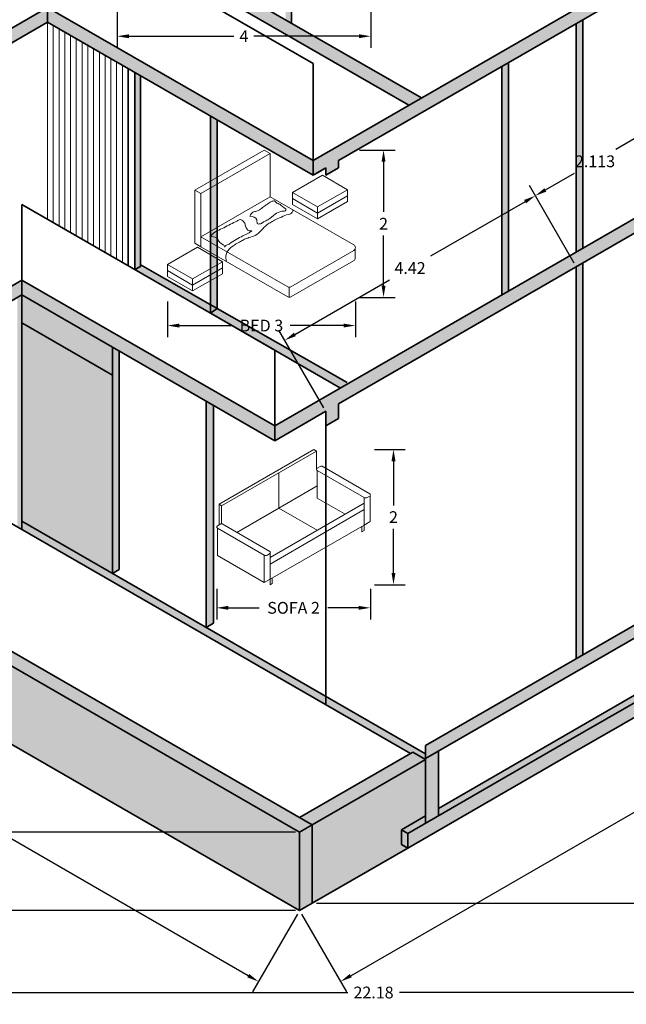
# Model space of a CAD drawing. Units: metres. Extents: x 26125 to 52281, y 14233 to 28508.
# Tile 2 of 4: x 26132.29 to 26141.57, y 14233.46 to 14248.53. Entities that reach past the tile are written whole.
import ezdxf

# ---------------------------------------------------------------- set-up
doc = ezdxf.new("R2010")
doc.units = ezdxf.units.M
for name, color, linetype, lineweight in [('A-ANNO-DIMS', 2, 'Continuous', 18), ('A-ELEV-CLAD', 30, 'Continuous', 13), ('A-ELEV-PATT', 32, 'Continuous', 13), ('A-FURN', 8, 'Continuous', 18), ('A-WALL', 7, 'Continuous', 35), ('A-WALL-PATT', 9, 'Continuous', 13)]:
    doc.layers.add(name, color=color, linetype=linetype, lineweight=lineweight)
doc.styles.get("Standard").update_dxf_attribs({"font": 'arial.ttf'})
doc.dimstyles.get("Standard").update_dxf_attribs({"dimtxt": 0.18, "dimasz": 0.18, "dimexe": 0.18, "dimexo": 0.0625, "dimgap": 0.09, "dimtad": 0, "dimtih": 1, "dimtoh": 1, "dimdec": 4, "dimzin": 0, "dimdsep": 46, "dimtxsty": 'Standard', "dimcen": 0.09, "dimadec": 0, "dimazin": 0, "dimtfac": 1, "dimtdec": 4, "dimtofl": 0, "dimtmove": 0, "dimatfit": 3, "dimfxl": 1, "dimtolj": 1, "dimtzin": 0, "dimarcsym": 0})

# ---------------------------------------------------------------- blocks, each defined once
blk = doc.blocks.new('SOFA')
for p, q in [((26137.785, 14240.572), (26139.234, 14241.408)), ((26137.821, 14240.543), (26139.277, 14241.383)), ((26139.277, 14241.383), (26139.234, 14241.408)), ((26139.277, 14241.103), (26139.277, 14241.383)), ((26138.697, 14241.049), (26138.697, 14240.509)), ((26139.287, 14241.121), (26139.34, 14241.151)), ((26139.287, 14241.086), (26140.002, 14240.673)), ((26139.287, 14241.086), (26139.287, 14240.664)), ((26139.36, 14241.151), (26140.09, 14240.73)), ((26138.697, 14240.509), (26139.287, 14240.85)), ((26138.566, 14239.754), (26140.002, 14240.587)), ((26139.712, 14240.419), (26139.287, 14240.664)), ((26140.002, 14240.673), (26140.002, 14240.251)), ((26140.052, 14240.673), (26140.09, 14240.695)), ((26140.095, 14240.699), (26140.095, 14240.305)), ((26137.785, 14240.253), (26137.785, 14240.572)), ((26137.821, 14240.543), (26137.785, 14240.572)), ((26137.821, 14240.271), (26137.821, 14240.543)), ((26138.697, 14240.509), (26138.056, 14240.139)), ((26138.566, 14239.654), (26140.002, 14240.487)), ((26139.284, 14240.17), (26138.697, 14240.509)), ((26140.002, 14240.251), (26140.095, 14240.305)), ((26137.759, 14240.238), (26137.811, 14240.269)), ((26137.759, 14240.204), (26138.474, 14239.791)), ((26137.759, 14240.204), (26137.759, 14239.782)), ((26137.831, 14240.269), (26138.561, 14239.847)), ((26138.566, 14239.422), (26140.002, 14240.251)), ((26139.969, 14240.147), (26139.969, 14240.232)), ((26140.002, 14240.166), (26139.969, 14240.147)), ((26140.002, 14240.251), (26140.002, 14240.166)), ((26138.474, 14239.369), (26137.759, 14239.782)), ((26138.474, 14239.791), (26138.474, 14239.369)), ((26138.524, 14239.791), (26138.561, 14239.813)), ((26138.566, 14239.817), (26138.566, 14239.422)), ((26138.474, 14239.369), (26138.566, 14239.422)), ((26138.566, 14239.336), (26138.566, 14239.421)), ((26138.598, 14239.44), (26138.598, 14239.355)), ((26138.598, 14239.355), (26138.566, 14239.336))]:
    blk.add_line(p, q)
for centre, radius, start, end in [((26139.297, 14241.103), 0.02, 120, 240), ((26139.35, 14241.134), 0.02, 60, 120), ((26140.027, 14240.716), 0.05, 240, 300), ((26140.08, 14240.712), 0.02, 300, 60), ((26137.769, 14240.221), 0.02, 120, 240), ((26137.821, 14240.251), 0.02, 60, 120), ((26138.551, 14239.83), 0.02, 300, 60), ((26138.499, 14239.834), 0.05, 240, 300)]:
    blk.add_arc(centre, radius, start, end)
blk = doc.blocks.new('BED')
for p, q in [((26136.061, 14245.293), (26137.122, 14245.905)), ((26137.216, 14245.851), (26137.122, 14245.905)), ((26136.155, 14245.238), (26137.216, 14245.851)), ((26137.216, 14245.191), (26137.216, 14245.851)), ((26137.556, 14245.257), (26138.013, 14245.521)), ((26138.013, 14245.521), (26138.397, 14245.298)), ((26136.061, 14244.478), (26136.061, 14245.293)), ((26136.061, 14245.293), (26136.155, 14245.238)), ((26137.94, 14245.035), (26137.556, 14245.257)), ((26137.556, 14245.257), (26137.556, 14245.163)), ((26138.397, 14245.298), (26137.94, 14245.035)), ((26138.397, 14245.298), (26138.397, 14245.205)), ((26136.155, 14244.578), (26136.155, 14245.238)), ((26136.155, 14244.578), (26137.216, 14245.191)), ((26138.493, 14244.454), (26137.216, 14245.191)), ((26137.94, 14244.941), (26137.556, 14245.163)), ((26137.556, 14245.163), (26137.556, 14245.073)), ((26138.397, 14245.205), (26137.94, 14244.941)), ((26138.397, 14245.115), (26137.94, 14244.851)), ((26138.397, 14245.205), (26138.397, 14245.115)), ((26137.94, 14244.851), (26137.556, 14245.073)), ((26137.94, 14245.035), (26137.94, 14244.941)), ((26137.94, 14244.941), (26137.94, 14244.851)), ((26136.155, 14244.578), (26137.482, 14243.813)), ((26136.155, 14244.578), (26136.155, 14244.423)), ((26135.644, 14244.153), (26136.101, 14244.416)), ((26136.155, 14244.423), (26136.061, 14244.478)), ((26136.101, 14244.416), (26136.485, 14244.194)), ((26136.155, 14244.423), (26137.482, 14243.657)), ((26137.532, 14243.813), (26138.493, 14244.367)), ((26138.516, 14244.4), (26138.516, 14244.255)), ((26137.532, 14243.657), (26138.491, 14244.211)), ((26136.028, 14243.931), (26135.644, 14244.153)), ((26135.644, 14244.153), (26135.644, 14244.059)), ((26136.028, 14243.837), (26135.644, 14244.059)), ((26135.644, 14244.059), (26135.644, 14243.969)), ((26136.485, 14244.194), (26136.028, 14243.931)), ((26136.485, 14244.101), (26136.028, 14243.837)), ((26136.485, 14244.194), (26136.485, 14244.101)), ((26136.485, 14244.101), (26136.485, 14244.011)), ((26136.028, 14243.747), (26135.644, 14243.969)), ((26136.485, 14244.011), (26136.028, 14243.747)), ((26136.028, 14243.931), (26136.028, 14243.837)), ((26136.028, 14243.837), (26136.028, 14243.747)), ((26137.507, 14243.806), (26137.507, 14243.651))]:
    blk.add_line(p, q)
for centre, start, end in [((26138.468, 14244.411), 300, 60), ((26138.466, 14244.255), 300, 0), ((26137.507, 14243.856), 240, 300), ((26137.507, 14243.701), 240, 300)]:
    blk.add_arc(centre, 0.05, start, end)
for points, knots in [([(26136.904, 14244.895), (26136.917, 14244.919), (26136.934, 14244.95), (26136.977, 14244.963), (26137.011, 14244.971), (26137.049, 14244.985), (26137.082, 14245.011), (26137.111, 14245.036), (26137.147, 14245.058), (26137.181, 14245.083), (26137.209, 14245.105), (26137.242, 14245.124), (26137.268, 14245.125), (26137.286, 14245.126)], [0, 0, 0, 0, 0.0750878, 0.0996797, 0.1335582, 0.1809259, 0.218328, 0.2572057, 0.2966137, 0.3461597, 0.3835693, 0.4042111, 0.458328, 0.458328, 0.458328, 0.458328]), ([(26137.286, 14245.126), (26137.295, 14245.113), (26137.312, 14245.088), (26137.347, 14245.084), (26137.372, 14245.065), (26137.395, 14245.048), (26137.416, 14245.03), (26137.429, 14245.018), (26137.44, 14245.013), (26137.448, 14245.01), (26137.451, 14245.008)], [0, 0, 0, 0, 0.0463958, 0.0840649, 0.098885, 0.1387133, 0.1705851, 0.1800712, 0.1936484, 0.2056105, 0.2056105, 0.2056105, 0.2056105]), ([(26136.545, 14244.198), (26136.538, 14244.236), (26136.524, 14244.317), (26136.621, 14244.433), (26136.731, 14244.486), (26136.822, 14244.54), (26136.896, 14244.569), (26137.037, 14244.602), (26137.116, 14244.737), (26137.232, 14244.804), (26137.304, 14244.843), (26137.393, 14244.882), (26137.475, 14244.919), (26137.554, 14244.93), (26137.563, 14244.986), (26137.572, 14244.985)], [0, 0, 0, 0, 0.109629, 0.235344, 0.413009, 0.480799, 0.550809, 0.653026, 0.903699, 0.971407, 1.0549, 1.149646, 1.262648, 1.330095, 1.369322, 1.369322, 1.369322, 1.369322]), ([(26137.072, 14244.773), (26137.086, 14244.784), (26137.118, 14244.81), (26137.2, 14244.845), (26137.282, 14244.923), (26137.366, 14244.971), (26137.457, 14244.968), (26137.453, 14244.999), (26137.451, 14245.008)], [0, 0, 0, 0, 0.0519704, 0.1236979, 0.2660086, 0.3781163, 0.4376787, 0.4619529, 0.4619529, 0.4619529, 0.4619529]), ([(26136.289, 14244.579), (26136.317, 14244.605), (26136.373, 14244.657), (26136.48, 14244.702), (26136.58, 14244.757), (26136.674, 14244.804), (26136.735, 14244.831), (26136.761, 14244.843)], [0, 0, 0, 0, 0.1136482, 0.2279116, 0.34476, 0.4564407, 0.5432537, 0.5432537, 0.5432537, 0.5432537]), ([(26136.761, 14244.843), (26136.784, 14244.83), (26136.826, 14244.806), (26136.834, 14244.729), (26136.874, 14244.666), (26136.918, 14244.666), (26136.932, 14244.666)], [0, 0, 0, 0, 0.0737944, 0.1363382, 0.222415, 0.2628991, 0.2628991, 0.2628991, 0.2628991]), ([(26136.904, 14244.895), (26136.951, 14244.888), (26137.024, 14244.876), (26137.007, 14244.768), (26137.048, 14244.774), (26137.062, 14244.773), (26137.072, 14244.773), (26137.072, 14244.773)], [0, 0, 0, 0, 0.1196046, 0.1868069, 0.2038069, 0.2293208, 0.231748, 0.231748, 0.231748, 0.231748]), ([(26136.521, 14244.42), (26136.525, 14244.428), (26136.538, 14244.451), (26136.572, 14244.454), (26136.652, 14244.515), (26136.766, 14244.579), (26136.886, 14244.634), (26136.928, 14244.663), (26136.932, 14244.666)], [0, 0, 0, 0, 0.0264518, 0.0758788, 0.090461, 0.3282148, 0.4667525, 0.4820056, 0.4820056, 0.4820056, 0.4820056]), ([(26136.289, 14244.579), (26136.328, 14244.581), (26136.388, 14244.583), (26136.424, 14244.511), (26136.465, 14244.471), (26136.509, 14244.448), (26136.518, 14244.426), (26136.521, 14244.42)], [0, 0, 0, 0, 0.1053267, 0.158497, 0.2248829, 0.2782536, 0.2973991, 0.2973991, 0.2973991, 0.2973991])]:
    blk.add_open_spline(points, degree=3, knots=knots)
blk = doc.blocks.new('*D4')
at = {"layer": 'A-ANNO-DIMS', "color": 0, "lineweight": -2, "transparency": 16777216}
for p, q in [((26134.548, 14244.218), (26134.548, 14243.67)), ((26137.422, 14244.218), (26137.422, 14243.67)), ((26134.728, 14243.85), (26135.547, 14243.85)), ((26137.242, 14243.85), (26136.424, 14243.85))]:
    blk.add_line(p, q, dxfattribs=at)
at = {"layer": 'A-ANNO-DIMS', "color": 0, "transparency": 16777216}
for points in [[(26134.728, 14243.88), (26134.728, 14243.82), (26134.548, 14243.85)], [(26137.242, 14243.88), (26137.242, 14243.82), (26137.422, 14243.85)]]:
    blk.add_solid(points, dxfattribs=at)
at = {"layer": 'Defpoints', "color": 0, "transparency": 16777216}
for p in [(26134.548, 14244.281), (26137.422, 14244.281), (26137.422, 14243.85)]:
    blk.add_point(p, dxfattribs=at)
at = {"layer": 'A-ANNO-DIMS', "color": 0, "transparency": 16777216, "insert": (26135.985, 14243.85), "char_height": 0.18, "attachment_point": 5}
blk.add_mtext('\\A1;BED 3', dxfattribs=at)
blk = doc.blocks.new('*D5')
at = {"layer": 'A-ANNO-DIMS', "color": 0, "lineweight": -2, "transparency": 16777216}
for p, q in [((26137.485, 14246.538), (26138.033, 14246.538)), ((26137.853, 14246.358), (26137.853, 14245.59)), ((26137.853, 14244.461), (26137.853, 14245.229)), ((26137.485, 14244.281), (26138.033, 14244.281))]:
    blk.add_line(p, q, dxfattribs=at)
at = {"layer": 'A-ANNO-DIMS', "color": 0, "transparency": 16777216}
for points in [[(26137.823, 14246.358), (26137.883, 14246.358), (26137.853, 14246.538)], [(26137.823, 14244.461), (26137.883, 14244.461), (26137.853, 14244.281)]]:
    blk.add_solid(points, dxfattribs=at)
at = {"layer": 'Defpoints', "color": 0, "transparency": 16777216}
for p in [(26137.422, 14246.538), (26137.853, 14246.538), (26137.422, 14244.281)]:
    blk.add_point(p, dxfattribs=at)
at = {"layer": 'A-ANNO-DIMS', "color": 0, "transparency": 16777216, "insert": (26137.853, 14245.409), "char_height": 0.18, "attachment_point": 5}
blk.add_mtext('\\A1;2', dxfattribs=at)
blk = doc.blocks.new('*D6')
at = {"layer": 'A-ANNO-DIMS', "color": 0, "lineweight": -2, "transparency": 16777216}
for p, q in [((26135.301, 14239.818), (26135.301, 14239.348)), ((26137.652, 14239.818), (26137.652, 14239.348)), ((26135.481, 14239.528), (26135.952, 14239.528)), ((26137.472, 14239.528), (26137.002, 14239.528))]:
    blk.add_line(p, q, dxfattribs=at)
at = {"layer": 'A-ANNO-DIMS', "color": 0, "transparency": 16777216}
for points in [[(26135.481, 14239.558), (26135.481, 14239.498), (26135.301, 14239.528)], [(26137.472, 14239.558), (26137.472, 14239.498), (26137.652, 14239.528)]]:
    blk.add_solid(points, dxfattribs=at)
at = {"layer": 'Defpoints', "color": 0, "transparency": 16777216}
for p in [(26135.301, 14239.881), (26137.652, 14239.881), (26137.652, 14239.528)]:
    blk.add_point(p, dxfattribs=at)
at = {"layer": 'A-ANNO-DIMS', "color": 0, "transparency": 16777216, "insert": (26136.477, 14239.528), "char_height": 0.18, "attachment_point": 5}
blk.add_mtext('\\A1;SOFA 2', dxfattribs=at)
blk = doc.blocks.new('*D7')
at = {"layer": 'A-ANNO-DIMS', "color": 0, "lineweight": -2, "transparency": 16777216}
for p, q in [((26137.715, 14241.953), (26138.185, 14241.953)), ((26138.005, 14241.773), (26138.005, 14241.097)), ((26138.005, 14240.061), (26138.005, 14240.737)), ((26137.715, 14239.881), (26138.185, 14239.881))]:
    blk.add_line(p, q, dxfattribs=at)
at = {"layer": 'A-ANNO-DIMS', "color": 0, "transparency": 16777216}
for points in [[(26137.975, 14241.773), (26138.035, 14241.773), (26138.005, 14241.953)], [(26137.975, 14240.061), (26138.035, 14240.061), (26138.005, 14239.881)]]:
    blk.add_solid(points, dxfattribs=at)
at = {"layer": 'Defpoints', "color": 0, "transparency": 16777216}
for p in [(26137.652, 14241.953), (26138.005, 14241.953), (26137.652, 14239.881)]:
    blk.add_point(p, dxfattribs=at)
at = {"layer": 'A-ANNO-DIMS', "color": 0, "transparency": 16777216, "insert": (26138.005, 14240.917), "char_height": 0.18, "attachment_point": 5}
blk.add_mtext('\\A1;2', dxfattribs=at)
blk = doc.blocks.new('*D9')
at = {"layer": 'A-ANNO-DIMS', "color": 0, "lineweight": -2, "transparency": 16777216}
for p, q in [((26133.777, 14248.964), (26133.777, 14248.1)), ((26137.657, 14248.964), (26137.657, 14248.1)), ((26133.957, 14248.28), (26135.565, 14248.28)), ((26137.477, 14248.28), (26135.869, 14248.28))]:
    blk.add_line(p, q, dxfattribs=at)
at = {"layer": 'A-ANNO-DIMS', "color": 0, "transparency": 16777216}
for points in [[(26133.957, 14248.31), (26133.957, 14248.25), (26133.777, 14248.28)], [(26137.477, 14248.31), (26137.477, 14248.25), (26137.657, 14248.28)]]:
    blk.add_solid(points, dxfattribs=at)
at = {"layer": 'Defpoints', "color": 0, "transparency": 16777216}
for p in [(26133.777, 14249.027), (26137.657, 14249.027), (26137.657, 14248.28)]:
    blk.add_point(p, dxfattribs=at)
at = {"layer": 'A-ANNO-DIMS', "color": 0, "transparency": 16777216, "insert": (26135.717, 14248.28), "char_height": 0.18, "attachment_point": 5}
blk.add_mtext('\\A1;4', dxfattribs=at)
blk = doc.blocks.new('*D10')
at = {"layer": 'A-ANNO-DIMS', "color": 0, "lineweight": -2, "transparency": 16777216}
for p, q in [((26148.791, 14241.887), (26148.791, 14233.458)), ((26126.609, 14240.579), (26126.609, 14233.458)), ((26126.789, 14233.638), (26137.305, 14233.638)), ((26148.611, 14233.638), (26138.096, 14233.638))]:
    blk.add_line(p, q, dxfattribs=at)
at = {"layer": 'A-ANNO-DIMS', "color": 0, "transparency": 16777216}
for points in [[(26126.789, 14233.668), (26126.789, 14233.608), (26126.609, 14233.638)], [(26148.611, 14233.668), (26148.611, 14233.608), (26148.791, 14233.638)]]:
    blk.add_solid(points, dxfattribs=at)
at = {"layer": 'Defpoints', "color": 0, "transparency": 16777216}
for p in [(26148.791, 14241.95), (26126.609, 14240.642), (26148.791, 14233.638)]:
    blk.add_point(p, dxfattribs=at)
at = {"layer": 'A-ANNO-DIMS', "color": 0, "transparency": 16777216, "insert": (26137.7, 14233.638), "char_height": 0.18, "attachment_point": 5}
blk.add_mtext('\\A1;22.18', dxfattribs=at)
blk = doc.blocks.new('*D11')
at = {"layer": 'A-ANNO-DIMS', "color": 0, "lineweight": -2, "transparency": 16777216}
for p, q in [((26141.524, 14258.813), (26150.226, 14258.813)), ((26150.046, 14258.633), (26150.046, 14247.091)), ((26150.046, 14235.186), (26150.046, 14246.727)), ((26136.826, 14235.006), (26150.226, 14235.006))]:
    blk.add_line(p, q, dxfattribs=at)
at = {"layer": 'A-ANNO-DIMS', "color": 0, "transparency": 16777216}
for points in [[(26150.016, 14258.633), (26150.076, 14258.633), (26150.046, 14258.813)], [(26150.016, 14235.186), (26150.076, 14235.186), (26150.046, 14235.006)]]:
    blk.add_solid(points, dxfattribs=at)
at = {"layer": 'Defpoints', "color": 0, "transparency": 16777216}
for p in [(26141.462, 14258.813), (26150.046, 14258.813), (26136.763, 14235.006)]:
    blk.add_point(p, dxfattribs=at)
at = {"layer": 'A-ANNO-DIMS', "color": 0, "transparency": 16777216, "insert": (26150.046, 14246.909), "char_height": 0.18, "attachment_point": 5}
blk.add_mtext('\\A1;23.807', dxfattribs=at)
blk = doc.blocks.new('*D12')
at = {"layer": 'A-ANNO-DIMS', "color": 0, "lineweight": -2, "transparency": 16777216}
for p, q in [((26126.578, 14240.588), (26125.892, 14239.399)), ((26126.138, 14239.465), (26130.646, 14236.862)), ((26135.784, 14233.896), (26131.276, 14236.498)), ((26136.536, 14234.838), (26135.85, 14233.65))]:
    blk.add_line(p, q, dxfattribs=at)
at = {"layer": 'A-ANNO-DIMS', "color": 0, "transparency": 16777216}
for points in [[(26126.153, 14239.491), (26126.123, 14239.439), (26125.982, 14239.555)], [(26135.799, 14233.922), (26135.769, 14233.87), (26135.94, 14233.806)]]:
    blk.add_solid(points, dxfattribs=at)
at = {"layer": 'Defpoints', "color": 0, "transparency": 16777216}
for p in [(26126.609, 14240.642), (26125.982, 14239.555), (26136.568, 14234.893)]:
    blk.add_point(p, dxfattribs=at)
at = {"layer": 'A-ANNO-DIMS', "color": 0, "transparency": 16777216, "insert": (26130.961, 14236.68), "char_height": 0.18, "attachment_point": 5}
blk.add_mtext('\\A1;11.499', dxfattribs=at)
blk = doc.blocks.new('*D13')
at = {"layer": 'A-ANNO-DIMS', "color": 0, "lineweight": -2, "transparency": 16777216}
for p, q in [((26148.822, 14241.896), (26149.508, 14240.707)), ((26149.262, 14240.773), (26143.619, 14237.515)), ((26137.351, 14233.896), (26142.994, 14237.154)), ((26136.599, 14234.838), (26137.285, 14233.65))]:
    blk.add_line(p, q, dxfattribs=at)
at = {"layer": 'A-ANNO-DIMS', "color": 0, "transparency": 16777216}
for points in [[(26149.247, 14240.799), (26149.277, 14240.747), (26149.418, 14240.863)], [(26137.336, 14233.922), (26137.366, 14233.87), (26137.195, 14233.806)]]:
    blk.add_solid(points, dxfattribs=at)
at = {"layer": 'Defpoints', "color": 0, "transparency": 16777216}
for p in [(26148.791, 14241.95), (26136.568, 14234.893), (26137.195, 14233.806)]:
    blk.add_point(p, dxfattribs=at)
at = {"layer": 'A-ANNO-DIMS', "color": 0, "transparency": 16777216, "insert": (26143.307, 14237.334), "char_height": 0.18, "attachment_point": 5}
blk.add_mtext('\\A1;14.114', dxfattribs=at)
blk = doc.blocks.new('*D14')
at = {"layer": 'A-ANNO-DIMS', "color": 0, "lineweight": -2, "transparency": 16777216}
for p, q in [((26136.505, 14236.093), (26125.173, 14236.093)), ((26125.353, 14235.913), (26125.353, 14235.673)), ((26125.353, 14235.073), (26125.353, 14235.312)), ((26136.505, 14234.893), (26125.173, 14234.893))]:
    blk.add_line(p, q, dxfattribs=at)
at = {"layer": 'A-ANNO-DIMS', "color": 0, "transparency": 16777216}
for points in [[(26125.323, 14235.913), (26125.383, 14235.913), (26125.353, 14236.093)], [(26125.323, 14235.073), (26125.383, 14235.073), (26125.353, 14234.893)]]:
    blk.add_solid(points, dxfattribs=at)
at = {"layer": 'Defpoints', "color": 0, "transparency": 16777216}
for p in [(26125.353, 14236.093), (26136.568, 14236.093), (26136.568, 14234.893)]:
    blk.add_point(p, dxfattribs=at)
at = {"layer": 'A-ANNO-DIMS', "color": 0, "transparency": 16777216, "insert": (26125.353, 14235.493), "char_height": 0.18, "attachment_point": 5}
blk.add_mtext('\\A1;1.2', dxfattribs=at)
blk = doc.blocks.new('*D29')
at = {"layer": 'A-ANNO-DIMS', "color": 0, "lineweight": -2, "transparency": 16777216}
for p, q in [((26140.77, 14244.804), (26140.083, 14245.993)), ((26140.018, 14245.747), (26138.57, 14244.911)), ((26136.498, 14243.715), (26137.946, 14244.551)), ((26136.939, 14242.592), (26136.253, 14243.781))]:
    blk.add_line(p, q, dxfattribs=at)
at = {"layer": 'A-ANNO-DIMS', "color": 0, "transparency": 16777216}
for points in [[(26140.003, 14245.773), (26140.033, 14245.721), (26140.173, 14245.837)], [(26136.483, 14243.741), (26136.513, 14243.689), (26136.343, 14243.625)]]:
    blk.add_solid(points, dxfattribs=at)
at = {"layer": 'Defpoints', "color": 0, "transparency": 16777216}
for p in [(26140.173, 14245.837), (26140.801, 14244.75), (26136.97, 14242.538)]:
    blk.add_point(p, dxfattribs=at)
at = {"layer": 'A-ANNO-DIMS', "color": 0, "transparency": 16777216, "insert": (26138.258, 14244.731), "char_height": 0.18, "attachment_point": 5}
blk.add_mtext('\\A1;4.42', dxfattribs=at)
blk = doc.blocks.new('*D30')
at = {"layer": 'A-ANNO-DIMS', "color": 0, "lineweight": -2, "transparency": 16777216}
for p, q in [((26142.6, 14245.861), (26141.913, 14247.049)), ((26141.847, 14246.803), (26141.404, 14246.547)), ((26140.329, 14245.927), (26140.773, 14246.183)), ((26140.77, 14244.804), (26140.083, 14245.993))]:
    blk.add_line(p, q, dxfattribs=at)
at = {"layer": 'A-ANNO-DIMS', "color": 0, "transparency": 16777216}
for points in [[(26141.832, 14246.829), (26141.862, 14246.777), (26142.003, 14246.893)], [(26140.314, 14245.953), (26140.344, 14245.901), (26140.173, 14245.837)]]:
    blk.add_solid(points, dxfattribs=at)
at = {"layer": 'Defpoints', "color": 0, "transparency": 16777216}
for p in [(26142.003, 14246.893), (26142.631, 14245.807), (26140.801, 14244.75)]:
    blk.add_point(p, dxfattribs=at)
at = {"layer": 'A-ANNO-DIMS', "color": 0, "transparency": 16777216, "insert": (26141.088, 14246.365), "char_height": 0.18, "attachment_point": 5}
blk.add_mtext('\\A1;2.113', dxfattribs=at)

msp = doc.modelspace()

# ---------------------------------------------------------------- hatches: boundary and pattern name
at = {"layer": 'A-ELEV-PATT'}
h = msp.add_hatch(color=256, dxfattribs=at)
h.dxf.hatch_style = 1
h.paths.add_polyline_path([(26139.7617, 14247.876), (26139.6635, 14247.8193), (26139.6635, 14244.3193), (26139.7617, 14244.376)])
h.paths.add_polyline_path([(26134.1363, 14247.6744), (26134.0497, 14247.7244), (26134.0497, 14244.7066), (26134.1363, 14244.7566)])
h.paths.add_polyline_path([(26135.2033, 14244.0405), (26135.3053, 14244.1136), (26135.3053, 14246.9994), (26135.2033, 14247.0583)])
h.paths.add_polyline_path([(26140.8009, 14238.75), (26140.8988, 14238.8065), (26140.8988, 14244.8065), (26140.8009, 14244.75)])
h.paths.add_polyline_path([(26142.7463, 14245.8732), (26142.6308, 14245.8065), (26142.6308, 14239.8065), (26142.7463, 14239.8732)])
h.paths.add_polyline_path([(26142.7463, 14249.5992), (26142.6308, 14249.5325), (26142.6308, 14246.0325), (26142.7463, 14246.0992)])
h.paths.add_polyline_path([(26140.8009, 14244.976), (26140.8988, 14245.0325), (26140.8988, 14248.5325), (26140.8009, 14248.476)])
h.paths.add_polyline_path([(26142.6308, 14249.7585), (26142.7463, 14249.8252), (26142.7463, 14253.3252), (26142.6308, 14253.2585)])
h.paths.add_polyline_path([(26136.4442, 14251.397), (26136.3576, 14251.447), (26136.3576, 14248.5341), (26136.4442, 14248.4841)])
h = msp.add_hatch(color=256, dxfattribs=at)
h.dxf.hatch_style = 1
h.paths.add_polyline_path([(26128.6368, 14249.6632), (26128.6368, 14249.4632), (26131.4647, 14247.8305), (26131.4647, 14248.0305)])
h.paths.add_polyline_path([(26129.6878, 14248.8564), (26129.5992, 14248.9076), (26129.5992, 14245.7744), (26129.6878, 14245.7232)])
h.paths.add_polyline_path([(26128.6368, 14249.4632), (26128.558, 14249.5087), (26128.558, 14246.2845), (26128.6368, 14246.33)])
h.paths.add_polyline_path([(26128.6368, 14249.6632), (26128.558, 14249.7087), (26128.558, 14249.5087), (26128.6368, 14249.4632)])
h.paths.add_polyline_path([(26128.6368, 14252.3748), (26128.558, 14252.4203), (26128.558, 14249.7087), (26128.6368, 14249.6632)])
h.paths.add_polyline_path([(26128.651, 14245.2941), (26128.5813, 14245.3344), (26128.5813, 14241.8829), (26128.651, 14241.9232)])
h.paths.add_polyline_path([(26128.651, 14241.9232), (26128.5813, 14241.8829), (26129.4364, 14241.3893), (26129.4364, 14241.4697)])
h.paths.add_polyline_path([(26129.4797, 14241.4143), (26129.4364, 14241.3893), (26130.2914, 14240.8956), (26130.2914, 14240.9456)])
h.paths.add_polyline_path([(26130.3373, 14240.9221), (26130.2914, 14240.8956), (26131.1464, 14240.402), (26131.1464, 14240.455)])
h.paths.add_polyline_path([(26130.3373, 14244.3206), (26130.2914, 14244.3471), (26130.2914, 14240.8956), (26130.3373, 14240.9221)])
h.paths.add_polyline_path([(26129.4797, 14244.8157), (26129.4364, 14244.8407), (26129.4364, 14241.3893), (26129.4797, 14241.4143)])
h.paths.add_polyline_path([(26135.2508, 14242.6282), (26135.1411, 14242.6915), (26135.1411, 14239.2275), (26135.2508, 14239.2908)])
h.paths.add_polyline_path([(26133.8091, 14243.4606), (26133.706, 14243.5201), (26133.706, 14240.056), (26133.8091, 14240.1155)])
h.paths.add_polyline_path([(26132.3223, 14244.3189), (26132.2523, 14244.2785), (26132.2523, 14240.7692), (26132.3223, 14240.7288)])
h = msp.add_hatch(color=256, dxfattribs=at)
h.dxf.hatch_style = 1
h.paths.add_polyline_path([(26135.2033, 14244.0405), (26135.2033, 14244.1685), (26134.1363, 14244.7566), (26134.0497, 14244.7066)])
h.paths.add_polyline_path([(26135.3042, 14244.1128), (26135.2033, 14244.0405), (26137.192, 14242.8924), (26137.2939, 14242.9679)])
h = msp.add_hatch(color=256, dxfattribs=at)
h.dxf.hatch_style = 1
h.paths.add_polyline_path([(26133.706, 14243.0916), (26132.3223, 14243.8904), (26132.3223, 14240.8549), (26133.706, 14240.056)])
h.paths.add_polyline_path([(26132.3223, 14244.3189), (26132.3223, 14243.8904), (26133.706, 14243.0916), (26133.706, 14243.5201)])
at = {"layer": 'A-WALL-PATT'}
h = msp.add_hatch(color=256, dxfattribs=at)
h.dxf.hatch_style = 1
h.paths.add_polyline_path([(26132.7127, 14248.4963), (26132.7127, 14248.7223), (26131.6604, 14248.1148), (26131.6604, 14247.8888)])
h.paths.add_polyline_path([(26132.7127, 14248.7223), (26132.7127, 14248.4963), (26136.7743, 14246.1513), (26136.7743, 14246.3773)])
h.paths.add_polyline_path([(26145.7774, 14251.3492), (26145.7774, 14250.8522), (26145.9732, 14250.9652), (26145.9732, 14251.6882), (26145.9732, 14252.3156), (26145.7774, 14252.4288), (26145.7774, 14251.5752), (26136.7743, 14246.3773), (26136.7743, 14246.1513), (26136.97, 14246.2643), (26136.97, 14246.1509), (26137.1658, 14246.2639), (26137.1658, 14246.3773)])
h.paths.add_polyline_path([(26135.3545, 14249.1132), (26135.1588, 14249.0002), (26138.2381, 14247.2224), (26138.4338, 14247.3354)])
h.paths.add_polyline_path([(26135.3545, 14252.0261), (26135.1588, 14252.1391), (26135.1588, 14249.0002), (26135.3545, 14249.1132)])
h.paths.add_polyline_path([(26137.9254, 14251.8375), (26137.7296, 14251.7245), (26137.7296, 14250.6548), (26137.9254, 14250.7678)], flags=17)
h.paths.add_polyline_path([(26144.9726, 14252.8939), (26144.9726, 14254.6106), (26144.7764, 14254.4973), (26144.7764, 14252.7806), (26145.7774, 14252.2026), (26145.7774, 14252.4288)])
h.paths.add_polyline_path([(26147.5095, 14248.6232), (26147.5095, 14242.6232), (26147.7052, 14242.7362), (26147.7052, 14248.9622), (26136.1883, 14242.3129), (26136.1883, 14242.0869), (26136.97, 14242.5383), (26136.97, 14242.3123), (26137.1658, 14242.4253), (26137.1658, 14242.6513)])
h.paths.add_polyline_path([(26145.9732, 14249.2872), (26145.7774, 14249.1742), (26145.7774, 14247.8492), (26145.9732, 14247.9622)], flags=17)
h.paths.add_polyline_path([(26145.5817, 14254.9622), (26145.5817, 14254.7362), (26145.7774, 14254.8492), (26145.7774, 14255.5272), (26145.5817, 14255.4142), (26145.5817, 14255.1882), (26141.4857, 14252.8234), (26141.4857, 14252.5974)])
h.paths.add_polyline_path([(26140.5667, 14258.3096), (26140.5667, 14258.0836), (26145.5817, 14255.1882), (26145.5817, 14255.4142)])
h.paths.add_polyline_path([(26140.7524, 14259.0772), (26140.7524, 14259.3025), (26137.3207, 14257.3212), (26137.5157, 14257.2086)])
h.paths.add_polyline_path([(26138.0751, 14255.9856), (26138.3349, 14256.1356), (26138.5947, 14255.9856), (26138.5947, 14256.5856), (26138.0751, 14256.2856), (26134.148, 14254.0183), (26134.4078, 14253.8683)])
h.paths.add_polyline_path([(26140.5667, 14258.0836), (26140.5667, 14258.3096), (26140.7524, 14258.4285), (26140.7524, 14259.0772), (26137.5157, 14257.2086), (26138.2834, 14256.7653)])
h.paths.add_polyline_path([(26145.1083, 14255.9136), (26145.0216, 14255.8636), (26144.9721, 14255.8922), (26144.9721, 14255.9922), (26144.9373, 14256.0123), (26144.8507, 14255.9623), (26144.8012, 14255.9909), (26144.8012, 14256.0909), (26144.7664, 14256.1109), (26144.6798, 14256.0609), (26144.6303, 14256.0896), (26144.6303, 14256.1896), (26144.5955, 14256.2096), (26144.5089, 14256.1596), (26144.4594, 14256.1882), (26144.4594, 14256.2882), (26144.4246, 14256.3083), (26144.338, 14256.2583), (26144.2885, 14256.2869), (26144.2885, 14256.3869), (26144.2537, 14256.407), (26144.1671, 14256.357), (26144.1176, 14256.3856), (26144.1176, 14256.4856), (26144.0828, 14256.5056), (26143.9962, 14256.4556), (26143.9466, 14256.4842), (26143.9466, 14256.5842), (26143.9119, 14256.6043), (26143.8253, 14256.5543), (26143.7757, 14256.5829), (26143.7757, 14256.6829), (26143.741, 14256.703), (26143.6544, 14256.653), (26143.6048, 14256.6816), (26143.6048, 14256.7816), (26143.5701, 14256.8017), (26143.4835, 14256.7517), (26143.4339, 14256.7803), (26143.4339, 14256.8803), (26143.3992, 14256.9003), (26143.3126, 14256.8503), (26143.263, 14256.8789), (26143.263, 14256.9789), (26143.2283, 14256.999), (26143.1417, 14256.949), (26143.0921, 14256.9776), (26143.0921, 14257.0776), (26143.0573, 14257.0977), (26142.9707, 14257.0477), (26142.9212, 14257.0763), (26142.9212, 14257.1763), (26142.8864, 14257.1964), (26142.7998, 14257.1464), (26142.7503, 14257.175), (26142.7503, 14257.275), (26142.7155, 14257.295), (26142.6289, 14257.245), (26142.5794, 14257.2736), (26142.5794, 14257.3736), (26142.5446, 14257.3937), (26142.458, 14257.3437), (26142.4085, 14257.3723), (26142.4085, 14257.4723), (26142.3737, 14257.4924), (26142.2871, 14257.4424), (26142.2376, 14257.471), (26142.2376, 14257.571), (26142.2322, 14257.5741), (26142.1456, 14257.5241), (26142.0961, 14257.5527), (26142.0961, 14257.6527), (26142.0613, 14257.6727), (26141.9747, 14257.6227), (26141.9252, 14257.6514), (26141.9252, 14257.7514), (26141.8904, 14257.7714), (26141.8038, 14257.7214), (26141.7542, 14257.75), (26141.7542, 14257.85), (26141.7195, 14257.8701), (26141.6329, 14257.8201), (26141.5833, 14257.8487), (26141.5833, 14257.9487), (26141.5486, 14257.9688), (26141.462, 14257.9188), (26141.4124, 14257.9474), (26141.4124, 14258.0474), (26141.3777, 14258.0674), (26141.2911, 14258.0174), (26141.2415, 14258.0461), (26141.2415, 14258.1461), (26141.2068, 14258.1661), (26141.1202, 14258.1161), (26141.0706, 14258.1447), (26141.0706, 14258.2447), (26141.0359, 14258.2648), (26140.9493, 14258.2148), (26140.8997, 14258.2434), (26140.8997, 14258.3434), (26140.8885, 14258.3499), (26140.8019, 14258.2999), (26140.7524, 14258.3285), (26140.7524, 14258.4285), (26140.5667, 14258.3096), (26145.5817, 14255.4142), (26145.7774, 14255.5272)])
h.paths.add_polyline_path([(26141.4857, 14254.3165), (26141.3093, 14254.2146), (26141.3093, 14252.4955), (26141.4857, 14252.5974)])
h.paths.add_polyline_path([(26140.2525, 14255.0285), (26140.0568, 14254.9155), (26141.29, 14254.2035), (26141.4857, 14254.3165)])
h = msp.add_hatch(color=256, dxfattribs=at)
h.dxf.hatch_style = 1
h.paths.add_polyline_path([(26126.9422, 14241.8758), (26126.7465, 14241.7628), (26136.5676, 14236.0925), (26136.7633, 14236.2055)])
h.paths.add_polyline_path([(26126.7465, 14241.7628), (26126.7318, 14241.7712), (26126.7318, 14244.7755), (26126.6095, 14244.8461), (26126.6095, 14240.6418), (26136.5676, 14234.8925), (26136.5676, 14236.0925)])
h.paths.add_polyline_path([(26138.4953, 14236.3449), (26138.4953, 14237.2055), (26136.7633, 14236.2055), (26136.7633, 14235.0055), (26138.2239, 14235.8488), (26138.1257, 14235.9055), (26138.1257, 14236.1315)])
h.paths.add_polyline_path([(26140.7034, 14237.2803), (26147.9009, 14241.4358), (26147.9009, 14241.6618), (26147.7052, 14241.5488), (26140.6052, 14237.4496), (26138.2239, 14236.0748), (26138.2239, 14235.8488)])
h.paths.add_polyline_path([(26140.6052, 14237.4496), (26142.2637, 14238.4072), (26142.2637, 14238.5206), (26138.6911, 14236.4579), (26138.6911, 14236.3445)], flags=17)
h.paths.add_polyline_path([(26138.4953, 14236.2315), (26138.4953, 14236.3449), (26138.1257, 14236.1315), (26138.2239, 14236.0748)], flags=17)
h.paths.add_polyline_path([(26138.2239, 14236.0748), (26138.1257, 14236.1315), (26138.1257, 14235.9055), (26138.2239, 14235.8488)], flags=17)
h.paths.add_polyline_path([(26136.7633, 14236.2055), (26136.5676, 14236.0925), (26136.5676, 14234.8925), (26136.7633, 14235.0055)])
h.paths.add_polyline_path([(26138.4953, 14237.2055), (26138.2996, 14237.3185), (26136.5676, 14236.3185), (26136.7633, 14236.2055)])
h.paths.add_polyline_path([(26128.558, 14246.2845), (26128.2718, 14246.1192), (26131.4647, 14244.2758), (26131.4647, 14244.6063)])
h.paths.add_polyline_path([(26128.2234, 14245.6367), (26128.2234, 14245.7792), (26126.6095, 14244.8474), (26126.6095, 14244.8461), (26126.7318, 14244.7755)])
h = msp.add_hatch(color=256, dxfattribs=at)
h.dxf.hatch_style = 1
h.paths.add_polyline_path([(26132.3223, 14244.3189), (26132.3223, 14244.5449), (26131.6604, 14244.1628), (26131.6604, 14243.9368)])
h.paths.add_polyline_path([(26132.3223, 14244.5449), (26132.3223, 14244.3189), (26136.1883, 14242.0869), (26136.1883, 14242.3129)])
h.paths.add_polyline_path([(26132.3223, 14240.8549), (26132.3223, 14240.7288), (26136.97, 14238.0454), (26136.97, 14238.1715)])
h.paths.add_polyline_path([(26128.2234, 14242.0896), (26128.2234, 14241.9635), (26131.1464, 14240.2759), (26131.1464, 14240.402)])
h = msp.add_hatch(color=256, dxfattribs=at)
h.dxf.hatch_style = 1
h.paths.add_polyline_path([(26133.8091, 14243.4606), (26133.706, 14243.5201), (26133.706, 14240.056), (26133.8091, 14240.1155)])
h = msp.add_hatch(color=256, dxfattribs=at)
h.dxf.hatch_style = 1
h.paths.add_polyline_path([(26147.5095, 14242.4232), (26147.5095, 14241.5492), (26142.4594, 14238.6336), (26142.4594, 14238.5202), (26147.7052, 14241.5488), (26147.7052, 14242.5102), (26147.5095, 14242.6232), (26147.2961, 14242.5), (26142.7463, 14239.8732), (26142.7463, 14239.6732)])
h.paths.add_polyline_path([(26142.7463, 14239.6732), (26142.7463, 14239.8732), (26138.4953, 14237.4189), (26138.4953, 14237.2189)])
h.paths.add_polyline_path([(26142.4594, 14239.5076), (26142.2637, 14239.3946), (26142.2637, 14238.4072), (26142.4594, 14238.5202), (26142.4594, 14238.6336)], flags=17)
h.paths.add_polyline_path([(26138.6911, 14237.3319), (26138.4953, 14237.2189), (26138.4953, 14236.2315), (26138.6911, 14236.3445)])
h = msp.add_hatch(color=256, dxfattribs=at)
h.dxf.hatch_style = 1
h.paths.add_polyline_path([(26136.97, 14238.1715), (26136.97, 14238.0454), (26138.2643, 14237.2982), (26138.2996, 14237.3185), (26138.4953, 14237.2055), (26138.4953, 14237.2909)])

# ---------------------------------------------------------------- linework, layer by layer
at = {"layer": 'A-ELEV-CLAD'}
for p, q in [((26132.7127, 14248.4963), (26132.7127, 14245.4785)), ((26132.8007, 14248.4454), (26132.8007, 14245.4277)), ((26132.8888, 14248.3946), (26132.8888, 14245.3768)), ((26132.9769, 14248.3437), (26132.9769, 14245.326)), ((26133.065, 14248.2929), (26133.065, 14245.2751)), ((26133.153, 14248.242), (26133.153, 14245.2243)), ((26133.2411, 14248.1912), (26133.2411, 14245.1734)), ((26133.3292, 14248.1403), (26133.3292, 14245.1226)), ((26133.4173, 14248.0895), (26133.4173, 14245.0717)), ((26133.5053, 14248.0386), (26133.5053, 14245.0209)), ((26133.5934, 14247.9878), (26133.5934, 14244.97)), ((26133.6815, 14247.9369), (26133.6815, 14244.9192)), ((26133.7696, 14247.8861), (26133.7696, 14244.8683)), ((26133.8577, 14247.8352), (26133.8577, 14244.8175)), ((26133.9457, 14247.7844), (26133.9457, 14244.7666))]:
    msp.add_line(p, q, dxfattribs=at)
at = {"layer": 'A-WALL'}
for p, q in [((26136.7743, 14246.3773), (26145.7774, 14251.5752)), ((26136.4442, 14251.397), (26136.4442, 14248.4841)), ((26137.1658, 14246.3773), (26145.7774, 14251.3492)), ((26136.7743, 14247.8613), (26132.7127, 14250.2063)), ((26135.3545, 14249.1132), (26138.4338, 14247.3354)), ((26138.2381, 14247.2224), (26135.1588, 14249.0002)), ((26136.1883, 14242.3129), (26147.7052, 14248.9622)), ((26132.7127, 14248.7223), (26131.6604, 14248.1148)), ((26136.7743, 14246.3773), (26132.7127, 14248.7223)), ((26132.7127, 14248.7223), (26132.7127, 14248.4963)), ((26137.1658, 14242.6513), (26147.5095, 14248.6232)), ((26132.7127, 14248.4963), (26131.6604, 14247.8888)), ((26136.7743, 14246.1513), (26132.7127, 14248.4963)), ((26140.8009, 14244.976), (26140.8009, 14248.476)), ((26140.8988, 14245.0325), (26140.8988, 14248.5325)), ((26136.7743, 14246.3773), (26136.7743, 14247.8613)), ((26139.6635, 14244.3193), (26139.6635, 14247.8193)), ((26139.7617, 14244.376), (26139.7617, 14247.876)), ((26133.9457, 14247.7844), (26133.9457, 14244.7666)), ((26134.0497, 14247.7244), (26134.0497, 14244.7066)), ((26134.1363, 14247.6744), (26134.1363, 14244.7566)), ((26135.2033, 14247.0583), (26135.2033, 14244.0405)), ((26135.3053, 14246.9994), (26135.3053, 14244.1136)), ((26136.7743, 14246.3773), (26136.7743, 14246.1513)), ((26137.1658, 14246.2639), (26137.1658, 14246.3773)), ((26136.7743, 14246.1513), (26136.97, 14246.2643)), ((26136.8419, 14246.1903), (26136.97, 14246.2643)), ((26136.97, 14246.2643), (26136.97, 14246.1509)), ((26136.97, 14246.2643), (26136.97, 14246.1509)), ((26136.97, 14246.1509), (26137.1658, 14246.2639)), ((26132.3223, 14245.7039), (26136.1883, 14243.4719)), ((26132.3223, 14245.7039), (26132.3223, 14244.3189)), ((26132.3223, 14245.2158), (26132.3223, 14240.7288)), ((26140.8988, 14238.8065), (26140.8988, 14244.8065)), ((26134.0497, 14244.7066), (26134.1363, 14244.7566)), ((26134.1363, 14244.782), (26137.2939, 14242.9766)), ((26140.8009, 14238.75), (26140.8009, 14244.75)), ((26132.3223, 14244.5449), (26131.6604, 14244.1628)), ((26136.1883, 14242.3129), (26132.3223, 14244.5449)), ((26132.3223, 14244.3189), (26131.6604, 14243.9368)), ((26136.1883, 14242.0869), (26132.3223, 14244.3189)), ((26135.2033, 14244.0405), (26135.3053, 14244.1136)), ((26135.2033, 14244.0405), (26137.192, 14242.8924)), ((26132.3223, 14243.8904), (26133.706, 14243.0916)), ((26133.706, 14240.056), (26133.706, 14243.5201)), ((26133.8091, 14240.1155), (26133.8091, 14243.4606)), ((26136.1883, 14243.4719), (26136.1883, 14242.0869)), ((26135.1411, 14239.2275), (26135.1411, 14242.6915)), ((26135.2508, 14239.2908), (26135.2508, 14242.6282)), ((26137.1658, 14242.6513), (26137.1658, 14242.4253)), ((26137.1658, 14242.4253), (26137.1658, 14242.6513)), ((26136.97, 14242.5383), (26136.1883, 14242.0869)), ((26136.97, 14242.3123), (26136.97, 14242.5383)), ((26136.97, 14242.5383), (26136.97, 14242.3123)), ((26136.97, 14242.5383), (26136.97, 14238.0454)), ((26137.1658, 14242.4253), (26136.97, 14242.3123)), ((26138.4953, 14237.4189), (26147.2961, 14242.5)), ((26138.4953, 14237.2189), (26147.5095, 14242.4232)), ((26140.7034, 14237.2803), (26148.7909, 14241.9496)), ((26136.7633, 14236.2055), (26126.9422, 14241.8758)), ((26136.5676, 14236.0925), (26126.7318, 14241.7712)), ((26140.6052, 14237.4496), (26147.7052, 14241.5488)), ((26132.1266, 14240.8418), (26138.2643, 14237.2982)), ((26132.3223, 14240.8549), (26138.4953, 14237.2909)), ((26136.5676, 14234.8925), (26126.6095, 14240.6418)), ((26133.706, 14240.056), (26133.8091, 14240.1155)), ((26135.1411, 14239.2275), (26135.2508, 14239.2908)), ((26138.6911, 14236.4579), (26142.2637, 14238.5206)), ((26140.6052, 14237.4496), (26138.2239, 14236.0748)), ((26138.4953, 14237.4189), (26138.4953, 14236.2315)), ((26138.2996, 14237.3185), (26136.5676, 14236.3185)), ((26138.4953, 14237.2055), (26138.2996, 14237.3185)), ((26138.6911, 14237.3319), (26138.6911, 14236.3445)), ((26136.7633, 14236.2055), (26138.4953, 14237.2055)), ((26136.7633, 14236.2055), (26136.5676, 14236.0925)), ((26136.5676, 14236.0925), (26136.5676, 14234.8925)), ((26136.7633, 14235.0055), (26136.7633, 14236.2055)), ((26138.2239, 14236.0748), (26138.1257, 14236.1315)), ((26138.2239, 14235.8488), (26136.7633, 14235.0055)), ((26136.5676, 14234.8925), (26136.7633, 14235.0055))]:
    msp.add_line(p, q, dxfattribs=at)
for points in [[(26140.7034, 14237.2803), (26138.2239, 14235.8488)], [(26138.4953, 14236.3449), (26138.1257, 14236.1315)], [(26138.1257, 14236.1315), (26138.1257, 14235.9055), (26138.2239, 14235.8488), (26138.2239, 14236.0748)]]:
    msp.add_lwpolyline(points, dxfattribs=at)

# ---------------------------------------------------------------- block references
at = {"layer": 'A-FURN'}
for name, p in [('BED', (-1.0954, 0.6324)), ('SOFA', (-2.4476, 0.5449))]:
    msp.add_blockref(name, p, dxfattribs=at)

# ---------------------------------------------------------------- dimensions: what is measured, and where the dimension line sits
at = {"layer": 'A-ANNO-DIMS'}
for base, p1, p2, angle, override, picture, middle in [((26150.0459, 14258.8126), (26136.7633, 14235.0055), (26141.462, 14258.8126), 90, {"dimdec": 3, "dimlfac": 1, "dimrnd": 0, "dimzin": 0, "dimdsep": 46, "dimlunit": 2}, '*D11', (26150.0459, 14246.9091)), ((26142.0033, 14246.8934), (26140.8009, 14244.75), (26142.6308, 14245.8065), 30, {"dimdec": 3, "dimlfac": 1, "dimrnd": 0, "dimzin": 0, "dimdsep": 46, "dimlunit": 2}, '*D30', (26141.0884, 14246.3652)), ((26137.8534, 14246.5379), (26137.4223, 14244.2809), (26137.4223, 14246.5379), 90, {"dimdec": 0, "dimlfac": 1, "dimrnd": 0, "dimzin": 0, "dimdsep": 46, "dimlunit": 2}, '*D5', (26137.8534, 14245.4094)), ((26140.1734, 14245.8369), (26136.97, 14242.5383), (26140.8009, 14244.75), 30, {"dimdec": 2, "dimlfac": 1, "dimrnd": 0, "dimzin": 0, "dimdsep": 46, "dimlunit": 2}, '*D29', (26138.258, 14244.731)), ((26137.1951, 14233.8057), (26148.7909, 14241.9496), (26136.5676, 14234.8925), 210, {"dimdec": 3, "dimlfac": 1, "dimrnd": 0, "dimzin": 0, "dimdsep": 46, "dimlunit": 2}, '*D13', (26143.3067, 14237.3342)), ((26138.0049, 14241.9534), (26137.6523, 14239.8808), (26137.6523, 14241.9534), 90, {"dimdec": 0, "dimlfac": 1, "dimrnd": 0, "dimzin": 0, "dimdsep": 46, "dimlunit": 2}, '*D7', (26138.0049, 14240.9171)), ((26125.982, 14239.555), (26136.5676, 14234.8925), (26126.6095, 14240.6418), 150, {"dimdec": 3, "dimlfac": 1, "dimrnd": 0, "dimzin": 0, "dimdsep": 46, "dimlunit": 2}, '*D12', (26130.961, 14236.6803)), ((26125.3534, 14236.0925), (26136.5676, 14234.8925), (26136.5676, 14236.0925), 90, {"dimdec": 1, "dimlfac": 1, "dimrnd": 0, "dimzin": 0, "dimdsep": 46, "dimlunit": 2}, '*D14', (26125.3534, 14235.4925))]:
    dim = msp.add_linear_dim(base=base, p1=p1, p2=p2, angle=angle, dimstyle='Standard', override=override, dxfattribs=at)
    dim.commit()
    dim.dimension.update_dxf_attribs({"geometry": picture, "text_midpoint": middle})
for base, p1, p2, override, picture, middle in [((26137.657, 14248.2796), (26133.7771, 14249.0266), (26137.657, 14249.0266), {"dimdec": 0, "dimlfac": 1, "dimrnd": 0, "dimzin": 0, "dimdsep": 46, "dimlunit": 2}, '*D9', (26135.717, 14248.2796)), ((26148.7909, 14233.6375), (26126.6095, 14240.6418), (26148.7909, 14241.9496), {"dimdec": 2, "dimlfac": 1, "dimrnd": 0, "dimzin": 0, "dimdsep": 46, "dimlunit": 2}, '*D10', (26137.7002, 14233.6375))]:
    dim = msp.add_linear_dim(base=base, p1=p1, p2=p2, dimstyle='Standard', override=override, dxfattribs=at)
    dim.commit()
    dim.dimension.update_dxf_attribs({"geometry": picture, "text_midpoint": middle})
for base, p1, p2, text, picture, middle in [((26137.4223, 14243.8498), (26134.5481, 14244.2809), (26137.4223, 14244.2809), 'BED <>', '*D4', (26135.9852, 14243.8498)), ((26137.6523, 14239.5281), (26135.301, 14239.8808), (26137.6523, 14239.8808), 'SOFA <>', '*D6', (26136.4766, 14239.5281))]:
    dim = msp.add_linear_dim(base=base, p1=p1, p2=p2, text=text, dimstyle='Standard', override={"dimdec": 0, "dimlfac": 1, "dimrnd": 0, "dimzin": 0, "dimdsep": 46, "dimlunit": 2}, dxfattribs=at)
    dim.commit()
    dim.dimension.update_dxf_attribs({"geometry": picture, "text_midpoint": middle})

doc.saveas('drawing.dxf')
